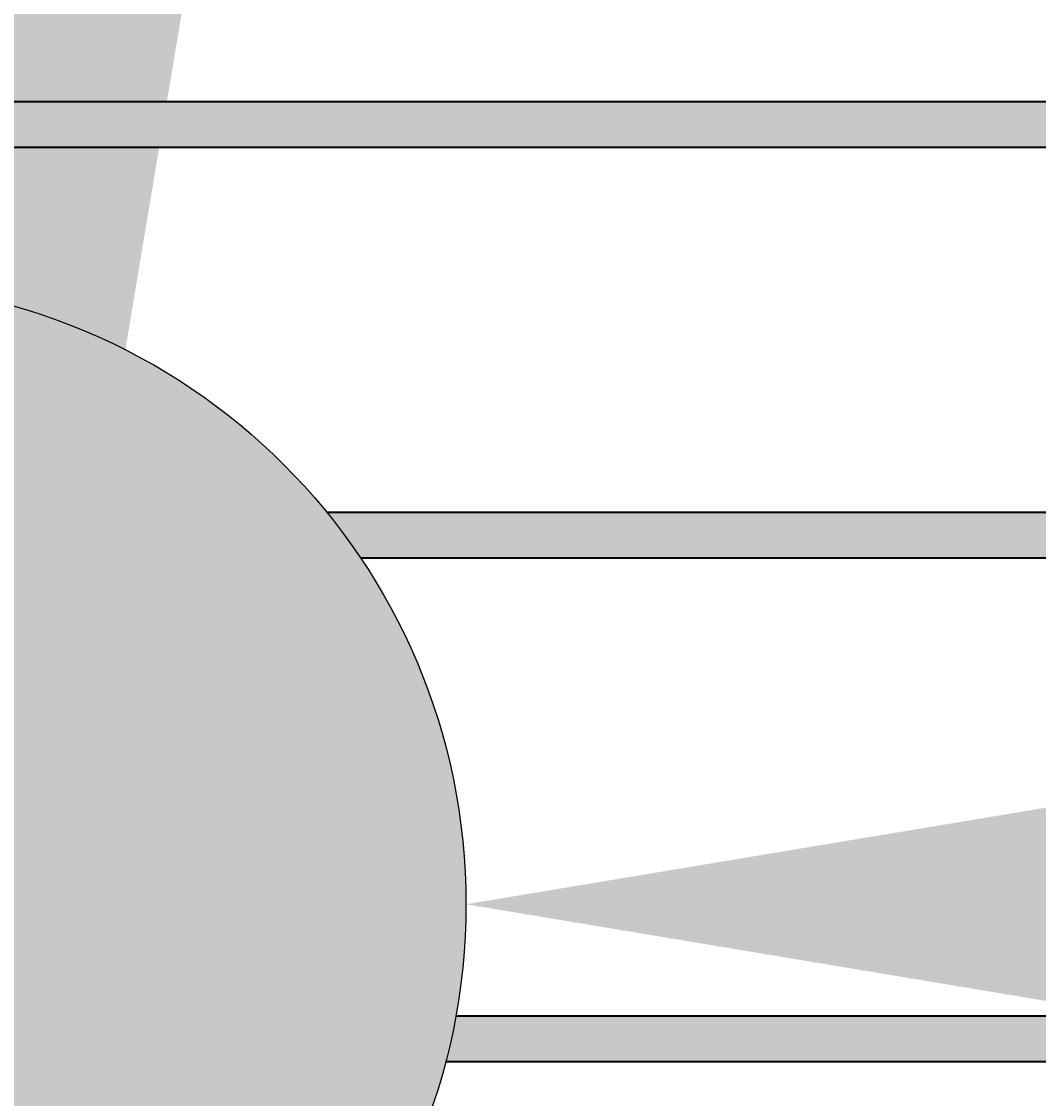
# Model space of a CAD drawing. Units: millimetres. Extents: x -22994 to 29398, y -19990 to 20176.
# Tile 19 of 135: x 54 to 77, y 76 to 99. Entities that reach past the tile are written whole.
import ezdxf

# ---------------------------------------------------------------- set-up
doc = ezdxf.new("R2010")
doc.units = ezdxf.units.MM
doc.header["$MEASUREMENT"] = 0
for name, color, linetype, lineweight in [('M-DIMS', 2, 'Continuous', 18), ('M-EQPM', 7, 'Continuous', 25), ('M-EQPM-PATT', 7, 'Continuous', 18), ('M-PIPE', 7, 'Continuous', 35)]:
    doc.layers.add(name, color=color, linetype=linetype, lineweight=lineweight)
doc.styles.get("Standard").update_dxf_attribs({"font": 'arial.ttf'})
doc.dimstyles.get("Standard").update_dxf_attribs({"dimtxt": 0.18, "dimasz": 10000, "dimexe": 0.18, "dimexo": 0.0625, "dimgap": 0.09, "dimtad": 0, "dimtih": 1, "dimtoh": 1, "dimdec": 0, "dimzin": 0, "dimdsep": 46, "dimtxsty": 'Standard', "dimcen": 0.09, "dimadec": 0, "dimazin": 0, "dimtfac": 1, "dimtdec": 0, "dimtofl": 0, "dimtmove": 0, "dimatfit": 3, "dimfxl": 1, "dimtolj": 1, "dimtzin": 0, "dimlwd": 30, "dimarcsym": 0})

# ---------------------------------------------------------------- blocks, each defined once
blk = doc.blocks.new('*D2')
at = {"layer": 'Defpoints', "color": 0, "transparency": 16777216}
for p in [(6.677, 10.271), (290.852, 10.271), (290.852, -5.079)]:
    blk.add_point(p, dxfattribs=at)
at = {"layer": 'M-DIMS', "color": 0, "lineweight": -2, "transparency": 16777216}
for p, q in [((6.677, 10.209), (6.677, -5.259)), ((290.852, 10.209), (290.852, -5.259))]:
    blk.add_line(p, q, dxfattribs=at)
at = {"layer": 'M-DIMS', "color": 0, "lineweight": 30, "transparency": 16777216}
for p, q in [((-9993.323, -5.079), (-19993.323, -5.079)), ((10290.852, -5.079), (20290.852, -5.079))]:
    blk.add_line(p, q, dxfattribs=at)
at = {"layer": 'M-DIMS', "color": 0, "transparency": 16777216}
for points in [[(-9993.323, 1661.588), (-9993.323, -1671.745), (6.677, -5.079)], [(10290.852, 1661.588), (10290.852, -1671.745), (290.852, -5.079)]]:
    blk.add_solid(points, dxfattribs=at)
at = {"layer": 'M-DIMS', "color": 0, "transparency": 16777216, "insert": (148.765, -5.079), "char_height": 0.18, "attachment_point": 5}
blk.add_mtext('\\A1;284.2', dxfattribs=at)
blk = doc.blocks.new('*D3')
at = {"layer": 'Defpoints', "color": 0, "transparency": 16777216}
for p in [(110.265, 204.165), (110.265, 176.366), (95.833, 127.967)]:
    blk.add_point(p, dxfattribs=at)
at = {"layer": 'M-DIMS', "color": 0, "lineweight": -2, "transparency": 16777216}
for p, q in [((95.833, 128.03), (95.833, 204.345)), ((110.265, 176.429), (110.265, 204.345))]:
    blk.add_line(p, q, dxfattribs=at)
at = {"layer": 'M-DIMS', "color": 0, "lineweight": 30, "transparency": 16777216}
for p, q in [((-9904.167, 204.165), (-19904.167, 204.165)), ((10110.265, 204.165), (20110.265, 204.165))]:
    blk.add_line(p, q, dxfattribs=at)
at = {"layer": 'M-DIMS', "color": 0, "transparency": 16777216}
for points in [[(-9904.167, 1870.832), (-9904.167, -1462.501), (95.833, 204.165)], [(10110.265, 1870.832), (10110.265, -1462.501), (110.265, 204.165)]]:
    blk.add_solid(points, dxfattribs=at)
at = {"layer": 'M-DIMS', "color": 0, "transparency": 16777216, "insert": (103.049, 204.165), "char_height": 0.18, "attachment_point": 5}
blk.add_mtext('\\A1;14.432', dxfattribs=at)
blk = doc.blocks.new('*D4')
at = {"layer": 'Defpoints', "color": 0, "transparency": 16777216}
for p in [(116.265, 204.165), (110.265, 176.366), (116.265, 176.366)]:
    blk.add_point(p, dxfattribs=at)
at = {"layer": 'M-DIMS', "color": 0, "lineweight": -2, "transparency": 16777216}
for p, q in [((110.265, 176.429), (110.265, 204.345)), ((116.265, 176.429), (116.265, 204.345))]:
    blk.add_line(p, q, dxfattribs=at)
at = {"layer": 'M-DIMS', "color": 0, "lineweight": 30, "transparency": 16777216}
for p, q in [((-9889.735, 204.165), (-19889.735, 204.165)), ((10116.265, 204.165), (20116.265, 204.165))]:
    blk.add_line(p, q, dxfattribs=at)
at = {"layer": 'M-DIMS', "color": 0, "transparency": 16777216}
for points in [[(-9889.735, 1870.832), (-9889.735, -1462.501), (110.265, 204.165)], [(10116.265, 1870.832), (10116.265, -1462.501), (116.265, 204.165)]]:
    blk.add_solid(points, dxfattribs=at)
at = {"layer": 'M-DIMS', "color": 0, "transparency": 16777216, "insert": (113.265, 204.165), "char_height": 0.18, "attachment_point": 5}
blk.add_mtext('\\A1;6', dxfattribs=at)
blk = doc.blocks.new('*D5')
at = {"layer": 'Defpoints', "color": 0, "transparency": 16777216}
for p in [(181.265, 204.165), (116.265, 176.366), (181.265, 176.366)]:
    blk.add_point(p, dxfattribs=at)
at = {"layer": 'M-DIMS', "color": 0, "lineweight": -2, "transparency": 16777216}
for p, q in [((116.265, 176.429), (116.265, 204.345)), ((181.265, 176.429), (181.265, 204.345))]:
    blk.add_line(p, q, dxfattribs=at)
at = {"layer": 'M-DIMS', "color": 0, "lineweight": 30, "transparency": 16777216}
for p, q in [((-9883.735, 204.165), (-19883.735, 204.165)), ((10181.265, 204.165), (20181.265, 204.165))]:
    blk.add_line(p, q, dxfattribs=at)
at = {"layer": 'M-DIMS', "color": 0, "transparency": 16777216}
for points in [[(-9883.735, 1870.832), (-9883.735, -1462.501), (116.265, 204.165)], [(10181.265, 1870.832), (10181.265, -1462.501), (181.265, 204.165)]]:
    blk.add_solid(points, dxfattribs=at)
at = {"layer": 'M-DIMS', "color": 0, "transparency": 16777216, "insert": (148.765, 204.165), "char_height": 0.18, "attachment_point": 5}
blk.add_mtext('\\A1;65', dxfattribs=at)
blk = doc.blocks.new('*D6')
at = {"layer": 'Defpoints', "color": 0, "transparency": 16777216}
for p in [(187.265, 204.165), (181.265, 176.366), (187.265, 176.366)]:
    blk.add_point(p, dxfattribs=at)
at = {"layer": 'M-DIMS', "color": 0, "lineweight": -2, "transparency": 16777216}
for p, q in [((181.265, 176.429), (181.265, 204.345)), ((187.265, 176.429), (187.265, 204.345))]:
    blk.add_line(p, q, dxfattribs=at)
at = {"layer": 'M-DIMS', "color": 0, "lineweight": 30, "transparency": 16777216}
for p, q in [((-9818.735, 204.165), (-19818.735, 204.165)), ((10187.265, 204.165), (20187.265, 204.165))]:
    blk.add_line(p, q, dxfattribs=at)
at = {"layer": 'M-DIMS', "color": 0, "transparency": 16777216}
for points in [[(-9818.735, 1870.832), (-9818.735, -1462.501), (181.265, 204.165)], [(10187.265, 1870.832), (10187.265, -1462.501), (187.265, 204.165)]]:
    blk.add_solid(points, dxfattribs=at)
at = {"layer": 'M-DIMS', "color": 0, "transparency": 16777216, "insert": (184.265, 204.165), "char_height": 0.18, "attachment_point": 5}
blk.add_mtext('\\A1;6', dxfattribs=at)
blk = doc.blocks.new('*D7')
at = {"layer": 'Defpoints', "color": 0, "transparency": 16777216}
for p in [(201.697, 204.165), (187.265, 176.366), (201.697, 127.967)]:
    blk.add_point(p, dxfattribs=at)
at = {"layer": 'M-DIMS', "color": 0, "lineweight": -2, "transparency": 16777216}
for p, q in [((187.265, 176.429), (187.265, 204.345)), ((201.697, 128.03), (201.697, 204.345))]:
    blk.add_line(p, q, dxfattribs=at)
at = {"layer": 'M-DIMS', "color": 0, "lineweight": 30, "transparency": 16777216}
for p, q in [((-9812.735, 204.165), (-19812.735, 204.165)), ((10201.697, 204.165), (20201.697, 204.165))]:
    blk.add_line(p, q, dxfattribs=at)
at = {"layer": 'M-DIMS', "color": 0, "transparency": 16777216}
for points in [[(-9812.735, 1870.832), (-9812.735, -1462.501), (187.265, 204.165)], [(10201.697, 1870.832), (10201.697, -1462.501), (201.697, 204.165)]]:
    blk.add_solid(points, dxfattribs=at)
at = {"layer": 'M-DIMS', "color": 0, "transparency": 16777216, "insert": (194.481, 204.165), "char_height": 0.18, "attachment_point": 5}
blk.add_mtext('\\A1;14.432', dxfattribs=at)
blk = doc.blocks.new('*D8')
at = {"layer": 'Defpoints', "color": 0, "transparency": 16777216}
for p in [(227.648, 204.165), (227.648, 146.73), (201.697, 127.967)]:
    blk.add_point(p, dxfattribs=at)
at = {"layer": 'M-DIMS', "color": 0, "lineweight": -2, "transparency": 16777216}
for p, q in [((201.697, 128.03), (201.697, 204.345)), ((227.648, 146.792), (227.648, 204.345))]:
    blk.add_line(p, q, dxfattribs=at)
at = {"layer": 'M-DIMS', "color": 0, "lineweight": 30, "transparency": 16777216}
for p, q in [((-9798.303, 204.165), (-19798.303, 204.165)), ((10227.648, 204.165), (20227.648, 204.165))]:
    blk.add_line(p, q, dxfattribs=at)
at = {"layer": 'M-DIMS', "color": 0, "transparency": 16777216}
for points in [[(-9798.303, 1870.832), (-9798.303, -1462.501), (201.697, 204.165)], [(10227.648, 1870.832), (10227.648, -1462.501), (227.648, 204.165)]]:
    blk.add_solid(points, dxfattribs=at)
at = {"layer": 'M-DIMS', "color": 0, "transparency": 16777216, "insert": (214.673, 204.165), "char_height": 0.18, "attachment_point": 5}
blk.add_mtext('\\A1;25.95', dxfattribs=at)
blk = doc.blocks.new('*D9')
at = {"layer": 'Defpoints', "color": 0, "transparency": 16777216}
for p in [(187.265, 176.366), (306.202, 176.366), (290.852, 10.271)]:
    blk.add_point(p, dxfattribs=at)
at = {"layer": 'M-DIMS', "color": 0, "lineweight": 30, "transparency": 16777216}
for p, q in [((306.202, 10176.366), (306.202, 20176.366)), ((306.202, -9989.729), (306.202, -19989.729))]:
    blk.add_line(p, q, dxfattribs=at)
at = {"layer": 'M-DIMS', "color": 0, "lineweight": -2, "transparency": 16777216}
for p, q in [((187.327, 176.366), (306.382, 176.366)), ((290.915, 10.271), (306.382, 10.271))]:
    blk.add_line(p, q, dxfattribs=at)
at = {"layer": 'M-DIMS', "color": 0, "transparency": 16777216}
for points in [[(-1360.465, 10176.366), (1972.869, 10176.366), (306.202, 176.366)], [(-1360.465, -9989.729), (1972.869, -9989.729), (306.202, 10.271)]]:
    blk.add_solid(points, dxfattribs=at)
at = {"layer": 'M-DIMS', "color": 0, "transparency": 16777216, "insert": (306.202, 93.319), "char_height": 0.18, "attachment_point": 5}
blk.add_mtext('\\A1;166.1', dxfattribs=at)
blk = doc.blocks.new('*D10')
at = {"layer": 'Defpoints', "color": 0, "transparency": 16777216}
for p in [(125.65, 136.071), (133.346, 136.071), (133.346, -5.079)]:
    blk.add_point(p, dxfattribs=at)
at = {"layer": 'M-DIMS', "color": 0, "lineweight": -2, "transparency": 16777216}
for p, q in [((125.65, 136.009), (125.65, -5.259)), ((133.346, 136.009), (133.346, -5.259))]:
    blk.add_line(p, q, dxfattribs=at)
at = {"layer": 'M-DIMS', "color": 0, "lineweight": 30, "transparency": 16777216}
for p, q in [((-9874.35, -5.079), (-19874.35, -5.079)), ((10133.346, -5.079), (20133.346, -5.079))]:
    blk.add_line(p, q, dxfattribs=at)
at = {"layer": 'M-DIMS', "color": 0, "transparency": 16777216}
for points in [[(-9874.35, 1661.588), (-9874.35, -1671.745), (125.65, -5.079)], [(10133.346, 1661.588), (10133.346, -1671.745), (133.346, -5.079)]]:
    blk.add_solid(points, dxfattribs=at)
at = {"layer": 'M-DIMS', "color": 0, "transparency": 16777216, "insert": (129.498, -5.079), "char_height": 0.18, "attachment_point": 5}
blk.add_mtext('\\A1;7.696', dxfattribs=at)
blk = doc.blocks.new('*D11')
at = {"layer": 'Defpoints', "color": 0, "transparency": 16777216}
for p in [(133.346, 136.071), (135.65, 136.071), (135.65, -5.079)]:
    blk.add_point(p, dxfattribs=at)
at = {"layer": 'M-DIMS', "color": 0, "lineweight": -2, "transparency": 16777216}
for p, q in [((133.346, 136.009), (133.346, -5.259)), ((135.65, 136.009), (135.65, -5.259))]:
    blk.add_line(p, q, dxfattribs=at)
at = {"layer": 'M-DIMS', "color": 0, "lineweight": 30, "transparency": 16777216}
for p, q in [((-9866.654, -5.079), (-19866.654, -5.079)), ((10135.65, -5.079), (20135.65, -5.079))]:
    blk.add_line(p, q, dxfattribs=at)
at = {"layer": 'M-DIMS', "color": 0, "transparency": 16777216}
for points in [[(-9866.654, 1661.588), (-9866.654, -1671.745), (133.346, -5.079)], [(10135.65, 1661.588), (10135.65, -1671.745), (135.65, -5.079)]]:
    blk.add_solid(points, dxfattribs=at)
at = {"layer": 'M-DIMS', "color": 0, "transparency": 16777216, "insert": (134.498, -5.079), "char_height": 0.18, "attachment_point": 5}
blk.add_mtext('\\A1;2.304', dxfattribs=at)
blk = doc.blocks.new('*D12')
at = {"layer": 'Defpoints', "color": 0, "transparency": 16777216}
for p in [(135.65, 136.071), (145.65, 136.071), (145.65, -5.079)]:
    blk.add_point(p, dxfattribs=at)
at = {"layer": 'M-DIMS', "color": 0, "lineweight": -2, "transparency": 16777216}
for p, q in [((135.65, 136.009), (135.65, -5.259)), ((145.65, 136.009), (145.65, -5.259))]:
    blk.add_line(p, q, dxfattribs=at)
at = {"layer": 'M-DIMS', "color": 0, "lineweight": 30, "transparency": 16777216}
for p, q in [((-9864.35, -5.079), (-19864.35, -5.079)), ((10145.65, -5.079), (20145.65, -5.079))]:
    blk.add_line(p, q, dxfattribs=at)
at = {"layer": 'M-DIMS', "color": 0, "transparency": 16777216}
for points in [[(-9864.35, 1661.588), (-9864.35, -1671.745), (135.65, -5.079)], [(10145.65, 1661.588), (10145.65, -1671.745), (145.65, -5.079)]]:
    blk.add_solid(points, dxfattribs=at)
at = {"layer": 'M-DIMS', "color": 0, "transparency": 16777216, "insert": (140.65, -5.079), "char_height": 0.18, "attachment_point": 5}
blk.add_mtext('\\A1;10', dxfattribs=at)
blk = doc.blocks.new('*D13')
at = {"layer": 'Defpoints', "color": 0, "transparency": 16777216}
for p in [(145.65, 136.071), (155.65, 136.071), (155.65, -5.079)]:
    blk.add_point(p, dxfattribs=at)
at = {"layer": 'M-DIMS', "color": 0, "lineweight": -2, "transparency": 16777216}
for p, q in [((145.65, 136.009), (145.65, -5.259)), ((155.65, 136.009), (155.65, -5.259))]:
    blk.add_line(p, q, dxfattribs=at)
at = {"layer": 'M-DIMS', "color": 0, "lineweight": 30, "transparency": 16777216}
for p, q in [((-9854.35, -5.079), (-19854.35, -5.079)), ((10155.65, -5.079), (20155.65, -5.079))]:
    blk.add_line(p, q, dxfattribs=at)
at = {"layer": 'M-DIMS', "color": 0, "transparency": 16777216}
for points in [[(-9854.35, 1661.588), (-9854.35, -1671.745), (145.65, -5.079)], [(10155.65, 1661.588), (10155.65, -1671.745), (155.65, -5.079)]]:
    blk.add_solid(points, dxfattribs=at)
at = {"layer": 'M-DIMS', "color": 0, "transparency": 16777216, "insert": (150.65, -5.079), "char_height": 0.18, "attachment_point": 5}
blk.add_mtext('\\A1;10', dxfattribs=at)
blk = doc.blocks.new('*D14')
at = {"layer": 'Defpoints', "color": 0, "transparency": 16777216}
for p in [(155.65, 136.071), (165.65, 136.071), (165.65, -5.079)]:
    blk.add_point(p, dxfattribs=at)
at = {"layer": 'M-DIMS', "color": 0, "lineweight": -2, "transparency": 16777216}
for p, q in [((155.65, 136.009), (155.65, -5.259)), ((165.65, 136.009), (165.65, -5.259))]:
    blk.add_line(p, q, dxfattribs=at)
at = {"layer": 'M-DIMS', "color": 0, "lineweight": 30, "transparency": 16777216}
for p, q in [((-9844.35, -5.079), (-19844.35, -5.079)), ((10165.65, -5.079), (20165.65, -5.079))]:
    blk.add_line(p, q, dxfattribs=at)
at = {"layer": 'M-DIMS', "color": 0, "transparency": 16777216}
for points in [[(-9844.35, 1661.588), (-9844.35, -1671.745), (155.65, -5.079)], [(10165.65, 1661.588), (10165.65, -1671.745), (165.65, -5.079)]]:
    blk.add_solid(points, dxfattribs=at)
at = {"layer": 'M-DIMS', "color": 0, "transparency": 16777216, "insert": (160.65, -5.079), "char_height": 0.18, "attachment_point": 5}
blk.add_mtext('\\A1;10', dxfattribs=at)
blk = doc.blocks.new('*D15')
at = {"layer": 'Defpoints', "color": 0, "transparency": 16777216}
for p in [(173.346, 154.788), (173.346, 136.071), (306.202, 136.071)]:
    blk.add_point(p, dxfattribs=at)
at = {"layer": 'M-DIMS', "color": 0, "lineweight": 30, "transparency": 16777216}
for p, q in [((306.202, 10154.788), (306.202, 20154.788)), ((306.202, -9863.929), (306.202, -19863.929))]:
    blk.add_line(p, q, dxfattribs=at)
at = {"layer": 'M-DIMS', "color": 0, "lineweight": -2, "transparency": 16777216}
for p, q in [((173.408, 154.788), (306.382, 154.788)), ((173.408, 136.071), (306.382, 136.071))]:
    blk.add_line(p, q, dxfattribs=at)
at = {"layer": 'M-DIMS', "color": 0, "transparency": 16777216}
for points in [[(-1360.465, 10154.788), (1972.869, 10154.788), (306.202, 154.788)], [(-1360.465, -9863.929), (1972.869, -9863.929), (306.202, 136.071)]]:
    blk.add_solid(points, dxfattribs=at)
at = {"layer": 'M-DIMS', "color": 0, "transparency": 16777216, "insert": (306.202, 145.43), "char_height": 0.18, "attachment_point": 5}
blk.add_mtext('\\A1;18.717', dxfattribs=at)
blk = doc.blocks.new('*D16')
at = {"layer": 'Defpoints', "color": 0, "transparency": 16777216}
for p in [(120.17, 204.165), (110.466, 48.035), (120.17, 48.035)]:
    blk.add_point(p, dxfattribs=at)
at = {"layer": 'M-DIMS', "color": 0, "lineweight": -2, "transparency": 16777216}
for p, q in [((110.466, 48.097), (110.466, 204.345)), ((120.17, 48.097), (120.17, 204.345))]:
    blk.add_line(p, q, dxfattribs=at)
at = {"layer": 'M-DIMS', "color": 0, "lineweight": 30, "transparency": 16777216}
for p, q in [((-9889.534, 204.165), (-19889.534, 204.165)), ((10120.17, 204.165), (20120.17, 204.165))]:
    blk.add_line(p, q, dxfattribs=at)
at = {"layer": 'M-DIMS', "color": 0, "transparency": 16777216}
for points in [[(-9889.534, 1870.832), (-9889.534, -1462.501), (110.466, 204.165)], [(10120.17, 1870.832), (10120.17, -1462.501), (120.17, 204.165)]]:
    blk.add_solid(points, dxfattribs=at)
at = {"layer": 'M-DIMS', "color": 0, "transparency": 16777216, "insert": (115.318, 204.165), "char_height": 0.18, "attachment_point": 5}
blk.add_mtext('\\A1;9.704', dxfattribs=at)
blk = doc.blocks.new('*D17')
at = {"layer": 'Defpoints', "color": 0, "transparency": 16777216}
for p in [(126.17, 204.165), (120.17, 48.035), (126.17, 48.035)]:
    blk.add_point(p, dxfattribs=at)
at = {"layer": 'M-DIMS', "color": 0, "lineweight": -2, "transparency": 16777216}
for p, q in [((120.17, 48.097), (120.17, 204.345)), ((126.17, 48.097), (126.17, 204.345))]:
    blk.add_line(p, q, dxfattribs=at)
at = {"layer": 'M-DIMS', "color": 0, "lineweight": 30, "transparency": 16777216}
for p, q in [((-9879.83, 204.165), (-19879.83, 204.165)), ((10126.17, 204.165), (20126.17, 204.165))]:
    blk.add_line(p, q, dxfattribs=at)
at = {"layer": 'M-DIMS', "color": 0, "transparency": 16777216}
for points in [[(-9879.83, 1870.832), (-9879.83, -1462.501), (120.17, 204.165)], [(10126.17, 1870.832), (10126.17, -1462.501), (126.17, 204.165)]]:
    blk.add_solid(points, dxfattribs=at)
at = {"layer": 'M-DIMS', "color": 0, "transparency": 16777216, "insert": (123.17, 204.165), "char_height": 0.18, "attachment_point": 5}
blk.add_mtext('\\A1;6', dxfattribs=at)
blk = doc.blocks.new('*D18')
at = {"layer": 'Defpoints', "color": 0, "transparency": 16777216}
for p in [(132.17, 204.165), (126.17, 48.035), (132.17, 48.035)]:
    blk.add_point(p, dxfattribs=at)
at = {"layer": 'M-DIMS', "color": 0, "lineweight": -2, "transparency": 16777216}
for p, q in [((126.17, 48.097), (126.17, 204.345)), ((132.17, 48.097), (132.17, 204.345))]:
    blk.add_line(p, q, dxfattribs=at)
at = {"layer": 'M-DIMS', "color": 0, "lineweight": 30, "transparency": 16777216}
for p, q in [((-9873.83, 204.165), (-19873.83, 204.165)), ((10132.17, 204.165), (20132.17, 204.165))]:
    blk.add_line(p, q, dxfattribs=at)
at = {"layer": 'M-DIMS', "color": 0, "transparency": 16777216}
for points in [[(-9873.83, 1870.832), (-9873.83, -1462.501), (126.17, 204.165)], [(10132.17, 1870.832), (10132.17, -1462.501), (132.17, 204.165)]]:
    blk.add_solid(points, dxfattribs=at)
at = {"layer": 'M-DIMS', "color": 0, "transparency": 16777216, "insert": (129.17, 204.165), "char_height": 0.18, "attachment_point": 5}
blk.add_mtext('\\A1;6', dxfattribs=at)
blk = doc.blocks.new('*D19')
at = {"layer": 'Defpoints', "color": 0, "transparency": 16777216}
for p in [(138.17, 204.165), (132.17, 48.035), (138.17, 48.035)]:
    blk.add_point(p, dxfattribs=at)
at = {"layer": 'M-DIMS', "color": 0, "lineweight": -2, "transparency": 16777216}
for p, q in [((132.17, 48.097), (132.17, 204.345)), ((138.17, 48.097), (138.17, 204.345))]:
    blk.add_line(p, q, dxfattribs=at)
at = {"layer": 'M-DIMS', "color": 0, "lineweight": 30, "transparency": 16777216}
for p, q in [((-9867.83, 204.165), (-19867.83, 204.165)), ((10138.17, 204.165), (20138.17, 204.165))]:
    blk.add_line(p, q, dxfattribs=at)
at = {"layer": 'M-DIMS', "color": 0, "transparency": 16777216}
for points in [[(-9867.83, 1870.832), (-9867.83, -1462.501), (132.17, 204.165)], [(10138.17, 1870.832), (10138.17, -1462.501), (138.17, 204.165)]]:
    blk.add_solid(points, dxfattribs=at)
at = {"layer": 'M-DIMS', "color": 0, "transparency": 16777216, "insert": (135.17, 204.165), "char_height": 0.18, "attachment_point": 5}
blk.add_mtext('\\A1;6', dxfattribs=at)
blk = doc.blocks.new('*D20')
at = {"layer": 'Defpoints', "color": 0, "transparency": 16777216}
for p in [(144.17, 204.165), (138.17, 48.035), (144.17, 48.035)]:
    blk.add_point(p, dxfattribs=at)
at = {"layer": 'M-DIMS', "color": 0, "lineweight": -2, "transparency": 16777216}
for p, q in [((138.17, 48.097), (138.17, 204.345)), ((144.17, 48.097), (144.17, 204.345))]:
    blk.add_line(p, q, dxfattribs=at)
at = {"layer": 'M-DIMS', "color": 0, "lineweight": 30, "transparency": 16777216}
for p, q in [((-9861.83, 204.165), (-19861.83, 204.165)), ((10144.17, 204.165), (20144.17, 204.165))]:
    blk.add_line(p, q, dxfattribs=at)
at = {"layer": 'M-DIMS', "color": 0, "transparency": 16777216}
for points in [[(-9861.83, 1870.832), (-9861.83, -1462.501), (138.17, 204.165)], [(10144.17, 1870.832), (10144.17, -1462.501), (144.17, 204.165)]]:
    blk.add_solid(points, dxfattribs=at)
at = {"layer": 'M-DIMS', "color": 0, "transparency": 16777216, "insert": (141.17, 204.165), "char_height": 0.18, "attachment_point": 5}
blk.add_mtext('\\A1;6', dxfattribs=at)
blk = doc.blocks.new('*D21')
at = {"layer": 'Defpoints', "color": 0, "transparency": 16777216}
for p in [(149.116, 204.165), (144.17, 48.035), (149.116, 48.035)]:
    blk.add_point(p, dxfattribs=at)
at = {"layer": 'M-DIMS', "color": 0, "lineweight": -2, "transparency": 16777216}
for p, q in [((144.17, 48.097), (144.17, 204.345)), ((149.116, 48.097), (149.116, 204.345))]:
    blk.add_line(p, q, dxfattribs=at)
at = {"layer": 'M-DIMS', "color": 0, "lineweight": 30, "transparency": 16777216}
for p, q in [((-9855.83, 204.165), (-19855.83, 204.165)), ((10149.116, 204.165), (20149.116, 204.165))]:
    blk.add_line(p, q, dxfattribs=at)
at = {"layer": 'M-DIMS', "color": 0, "transparency": 16777216}
for points in [[(-9855.83, 1870.832), (-9855.83, -1462.501), (144.17, 204.165)], [(10149.116, 1870.832), (10149.116, -1462.501), (149.116, 204.165)]]:
    blk.add_solid(points, dxfattribs=at)
at = {"layer": 'M-DIMS', "color": 0, "transparency": 16777216, "insert": (146.643, 204.165), "char_height": 0.18, "attachment_point": 5}
blk.add_mtext('\\A1;4.945', dxfattribs=at)
blk = doc.blocks.new('*D22')
at = {"layer": 'Defpoints', "color": 0, "transparency": 16777216}
for p in [(149.116, 30.99), (155.116, 30.99), (155.116, -5.079)]:
    blk.add_point(p, dxfattribs=at)
at = {"layer": 'M-DIMS', "color": 0, "lineweight": -2, "transparency": 16777216}
for p, q in [((149.116, 30.927), (149.116, -5.259)), ((155.116, 30.927), (155.116, -5.259))]:
    blk.add_line(p, q, dxfattribs=at)
at = {"layer": 'M-DIMS', "color": 0, "lineweight": 30, "transparency": 16777216}
for p, q in [((-9850.884, -5.079), (-19850.884, -5.079)), ((10155.116, -5.079), (20155.116, -5.079))]:
    blk.add_line(p, q, dxfattribs=at)
at = {"layer": 'M-DIMS', "color": 0, "transparency": 16777216}
for points in [[(-9850.884, 1661.588), (-9850.884, -1671.745), (149.116, -5.079)], [(10155.116, 1661.588), (10155.116, -1671.745), (155.116, -5.079)]]:
    blk.add_solid(points, dxfattribs=at)
at = {"layer": 'M-DIMS', "color": 0, "transparency": 16777216, "insert": (152.116, -5.079), "char_height": 0.18, "attachment_point": 5}
blk.add_mtext('\\A1;6', dxfattribs=at)
blk = doc.blocks.new('*D23')
at = {"layer": 'Defpoints', "color": 0, "transparency": 16777216}
for p in [(155.116, 30.99), (161.116, 30.99), (161.116, -5.079)]:
    blk.add_point(p, dxfattribs=at)
at = {"layer": 'M-DIMS', "color": 0, "lineweight": -2, "transparency": 16777216}
for p, q in [((155.116, 30.927), (155.116, -5.259)), ((161.116, 30.927), (161.116, -5.259))]:
    blk.add_line(p, q, dxfattribs=at)
at = {"layer": 'M-DIMS', "color": 0, "lineweight": 30, "transparency": 16777216}
for p, q in [((-9844.884, -5.079), (-19844.884, -5.079)), ((10161.116, -5.079), (20161.116, -5.079))]:
    blk.add_line(p, q, dxfattribs=at)
at = {"layer": 'M-DIMS', "color": 0, "transparency": 16777216}
for points in [[(-9844.884, 1661.588), (-9844.884, -1671.745), (155.116, -5.079)], [(10161.116, 1661.588), (10161.116, -1671.745), (161.116, -5.079)]]:
    blk.add_solid(points, dxfattribs=at)
at = {"layer": 'M-DIMS', "color": 0, "transparency": 16777216, "insert": (158.116, -5.079), "char_height": 0.18, "attachment_point": 5}
blk.add_mtext('\\A1;6', dxfattribs=at)
blk = doc.blocks.new('*D24')
at = {"layer": 'Defpoints', "color": 0, "transparency": 16777216}
for p in [(161.116, 30.99), (166.439, 30.99), (166.439, -5.079)]:
    blk.add_point(p, dxfattribs=at)
at = {"layer": 'M-DIMS', "color": 0, "lineweight": -2, "transparency": 16777216}
for p, q in [((161.116, 30.927), (161.116, -5.259)), ((166.439, 30.927), (166.439, -5.259))]:
    blk.add_line(p, q, dxfattribs=at)
at = {"layer": 'M-DIMS', "color": 0, "lineweight": 30, "transparency": 16777216}
for p, q in [((-9838.884, -5.079), (-19838.884, -5.079)), ((10166.439, -5.079), (20166.439, -5.079))]:
    blk.add_line(p, q, dxfattribs=at)
at = {"layer": 'M-DIMS', "color": 0, "transparency": 16777216}
for points in [[(-9838.884, 1661.588), (-9838.884, -1671.745), (161.116, -5.079)], [(10166.439, 1661.588), (10166.439, -1671.745), (166.439, -5.079)]]:
    blk.add_solid(points, dxfattribs=at)
at = {"layer": 'M-DIMS', "color": 0, "transparency": 16777216, "insert": (163.777, -5.079), "char_height": 0.18, "attachment_point": 5}
blk.add_mtext('\\A1;5.323', dxfattribs=at)
blk = doc.blocks.new('*D25')
at = {"layer": 'Defpoints', "color": 0, "transparency": 16777216}
for p in [(166.439, 30.99), (172.439, 30.99), (172.439, -5.079)]:
    blk.add_point(p, dxfattribs=at)
at = {"layer": 'M-DIMS', "color": 0, "lineweight": -2, "transparency": 16777216}
for p, q in [((166.439, 30.927), (166.439, -5.259)), ((172.439, 30.927), (172.439, -5.259))]:
    blk.add_line(p, q, dxfattribs=at)
at = {"layer": 'M-DIMS', "color": 0, "lineweight": 30, "transparency": 16777216}
for p, q in [((-9833.561, -5.079), (-19833.561, -5.079)), ((10172.439, -5.079), (20172.439, -5.079))]:
    blk.add_line(p, q, dxfattribs=at)
at = {"layer": 'M-DIMS', "color": 0, "transparency": 16777216}
for points in [[(-9833.561, 1661.588), (-9833.561, -1671.745), (166.439, -5.079)], [(10172.439, 1661.588), (10172.439, -1671.745), (172.439, -5.079)]]:
    blk.add_solid(points, dxfattribs=at)
at = {"layer": 'M-DIMS', "color": 0, "transparency": 16777216, "insert": (169.439, -5.079), "char_height": 0.18, "attachment_point": 5}
blk.add_mtext('\\A1;6', dxfattribs=at)
blk = doc.blocks.new('*D26')
at = {"layer": 'Defpoints', "color": 0, "transparency": 16777216}
for p in [(172.439, 30.99), (178.439, 30.99), (178.439, -5.079)]:
    blk.add_point(p, dxfattribs=at)
at = {"layer": 'M-DIMS', "color": 0, "lineweight": -2, "transparency": 16777216}
for p, q in [((172.439, 30.927), (172.439, -5.259)), ((178.439, 30.927), (178.439, -5.259))]:
    blk.add_line(p, q, dxfattribs=at)
at = {"layer": 'M-DIMS', "color": 0, "lineweight": 30, "transparency": 16777216}
for p, q in [((-9827.561, -5.079), (-19827.561, -5.079)), ((10178.439, -5.079), (20178.439, -5.079))]:
    blk.add_line(p, q, dxfattribs=at)
at = {"layer": 'M-DIMS', "color": 0, "transparency": 16777216}
for points in [[(-9827.561, 1661.588), (-9827.561, -1671.745), (172.439, -5.079)], [(10178.439, 1661.588), (10178.439, -1671.745), (178.439, -5.079)]]:
    blk.add_solid(points, dxfattribs=at)
at = {"layer": 'M-DIMS', "color": 0, "transparency": 16777216, "insert": (175.439, -5.079), "char_height": 0.18, "attachment_point": 5}
blk.add_mtext('\\A1;6', dxfattribs=at)
blk = doc.blocks.new('*D27')
at = {"layer": 'Defpoints', "color": 0, "transparency": 16777216}
for p in [(178.439, 30.99), (188.117, 30.99), (188.117, -5.079)]:
    blk.add_point(p, dxfattribs=at)
at = {"layer": 'M-DIMS', "color": 0, "lineweight": -2, "transparency": 16777216}
for p, q in [((178.439, 30.927), (178.439, -5.259)), ((188.117, 30.927), (188.117, -5.259))]:
    blk.add_line(p, q, dxfattribs=at)
at = {"layer": 'M-DIMS', "color": 0, "lineweight": 30, "transparency": 16777216}
for p, q in [((-9821.561, -5.079), (-19821.561, -5.079)), ((10188.117, -5.079), (20188.117, -5.079))]:
    blk.add_line(p, q, dxfattribs=at)
at = {"layer": 'M-DIMS', "color": 0, "transparency": 16777216}
for points in [[(-9821.561, 1661.588), (-9821.561, -1671.745), (178.439, -5.079)], [(10188.117, 1661.588), (10188.117, -1671.745), (188.117, -5.079)]]:
    blk.add_solid(points, dxfattribs=at)
at = {"layer": 'M-DIMS', "color": 0, "transparency": 16777216, "insert": (183.278, -5.079), "char_height": 0.18, "attachment_point": 5}
blk.add_mtext('\\A1;9.679', dxfattribs=at)
blk = doc.blocks.new('*D28')
at = {"layer": 'Defpoints', "color": 0, "transparency": 16777216}
for p in [(188.117, 48.035), (306.202, 48.035), (188.117, 30.99)]:
    blk.add_point(p, dxfattribs=at)
at = {"layer": 'M-DIMS', "color": 0, "lineweight": 30, "transparency": 16777216}
for p, q in [((306.202, 10048.035), (306.202, 20048.035)), ((306.202, -9969.01), (306.202, -19969.01))]:
    blk.add_line(p, q, dxfattribs=at)
at = {"layer": 'M-DIMS', "color": 0, "lineweight": -2, "transparency": 16777216}
for p, q in [((188.18, 48.035), (306.382, 48.035)), ((188.18, 30.99), (306.382, 30.99))]:
    blk.add_line(p, q, dxfattribs=at)
at = {"layer": 'M-DIMS', "color": 0, "transparency": 16777216}
for points in [[(-1360.465, 10048.035), (1972.869, 10048.035), (306.202, 48.035)], [(-1360.465, -9969.01), (1972.869, -9969.01), (306.202, 30.99)]]:
    blk.add_solid(points, dxfattribs=at)
at = {"layer": 'M-DIMS', "color": 0, "transparency": 16777216, "insert": (306.202, 39.512), "char_height": 0.18, "attachment_point": 5}
blk.add_mtext('\\A1;17.045', dxfattribs=at)
blk = doc.blocks.new('*D29')
at = {"layer": 'Defpoints', "color": 0, "transparency": 16777216}
for p in [(36.801, 80.045), (64.03, 80.045)]:
    blk.add_point(p, dxfattribs=at)
at = {"layer": 'M-DIMS', "color": 0, "lineweight": -2, "transparency": 16777216}
for p, q in [((50.325, 80.045), (50.505, 80.045)), ((50.415, 79.955), (50.415, 80.135))]:
    blk.add_line(p, q, dxfattribs=at)
at = {"layer": 'M-DIMS', "color": 0, "lineweight": 30, "transparency": 16777216}
blk.add_line((20064.03, 80.03), (10064.03, 80.038), dxfattribs=at)
at = {"layer": 'M-DIMS', "color": 0, "transparency": 16777216}
blk.add_solid([(10064.031, 1746.704), (10064.028, -1586.629), (64.03, 80.045)], dxfattribs=at)
at = {"layer": 'M-DIMS', "color": 0, "transparency": 16777216, "insert": (20064.521, 80.03), "char_height": 0.18, "attachment_point": 5}
blk.add_mtext('\\A1;∅27.23', dxfattribs=at)
blk = doc.blocks.new('*D32')
at = {"layer": 'Defpoints', "color": 0, "transparency": 16777216}
for p in [(57.164, 118.614), (52.413, 113.093)]:
    blk.add_point(p, dxfattribs=at)
at = {"layer": 'M-DIMS', "color": 0, "lineweight": -2, "transparency": 16777216}
for p, q in [((57.164, 118.524), (57.164, 118.704)), ((57.074, 118.614), (57.254, 118.614))]:
    blk.add_line(p, q, dxfattribs=at)
at = {"layer": 'M-DIMS', "color": 0, "lineweight": 30, "transparency": 16777216}
for p, q in [((-12992.534, -15047.031), (-6470.06, -7466.969)), ((-22992.534, -15047.031), (-12992.534, -15047.031))]:
    blk.add_line(p, q, dxfattribs=at)
at = {"layer": 'M-DIMS', "color": 0, "transparency": 16777216}
blk.add_solid([(-7733.404, -6379.89), (-5206.717, -8554.048), (52.413, 113.093)], dxfattribs=at)
at = {"layer": 'M-DIMS', "color": 0, "transparency": 16777216, "insert": (-22993.208, -15047.031), "char_height": 0.18, "attachment_point": 5}
blk.add_mtext('\\A1;2X R7.284', dxfattribs=at)
blk = doc.blocks.new('*D36')
at = {"layer": 'Defpoints', "color": 0, "transparency": 16777216}
for p in [(46.39, 31.303), (46.387, 26.593)]:
    blk.add_point(p, dxfattribs=at)
at = {"layer": 'M-DIMS', "color": 0, "lineweight": 30, "transparency": 16777216}
for p, q in [((57.15, 20031.301), (51.77, 10031.302)), ((10057.15, 20031.301), (57.15, 20031.301))]:
    blk.add_line(p, q, dxfattribs=at)
at = {"layer": 'M-DIMS', "color": 0, "lineweight": -2, "transparency": 16777216}
for p, q in [((46.389, 28.858), (46.389, 29.038)), ((46.299, 28.948), (46.479, 28.948))]:
    blk.add_line(p, q, dxfattribs=at)
at = {"layer": 'M-DIMS', "color": 0, "transparency": 16777216}
blk.add_solid([(-1614.896, 10032.199), (1718.436, 10030.405), (46.39, 31.303)], dxfattribs=at)
at = {"layer": 'M-DIMS', "color": 0, "transparency": 16777216, "insert": (10057.554, 20031.301), "char_height": 0.18, "attachment_point": 5}
blk.add_mtext('\\A1;∅4.71', dxfattribs=at)
blk = doc.blocks.new('*D37')
at = {"layer": 'Defpoints', "color": 0, "transparency": 16777216}
for p in [(54.834, 118.615), (59.494, 118.614)]:
    blk.add_point(p, dxfattribs=at)
at = {"layer": 'M-DIMS', "color": 0, "lineweight": -2, "transparency": 16777216}
for p, q in [((57.164, 118.524), (57.164, 118.704)), ((57.074, 118.614), (57.254, 118.614))]:
    blk.add_line(p, q, dxfattribs=at)
at = {"layer": 'M-DIMS', "color": 0, "lineweight": 30, "transparency": 16777216}
blk.add_line((20059.493, 116.253), (10059.494, 117.434), dxfattribs=at)
at = {"layer": 'M-DIMS', "color": 0, "transparency": 16777216}
blk.add_solid([(10059.69, 1784.1), (10059.297, -1549.233), (59.494, 118.614)], dxfattribs=at)
at = {"layer": 'M-DIMS', "color": 0, "transparency": 16777216, "insert": (20059.985, 116.253), "char_height": 0.18, "attachment_point": 5}
blk.add_mtext('\\A1;∅4.659', dxfattribs=at)

msp = doc.modelspace()

# ---------------------------------------------------------------- hatches: boundary and pattern name
at = {"layer": 'M-EQPM-PATT'}
h = msp.add_hatch(color=256, dxfattribs=at)
h.set_gradient(color1=(205, 32, 39), color2=(205, 32, 39), tint=1)
h.paths.add_polyline_path([(116.2647, 150.3662), (116.2647, 170.3662), (116.2647, 176.3662), (110.2647, 176.3662), (110.2647, 152.0276), (95.8327, 127.967), (95.8327, 16.6063), (201.6967, 16.6063), (201.6967, 127.967), (187.2647, 152.0276), (187.2647, 176.3662), (181.2647, 176.3662), (181.2647, 170.3662), (181.2647, 150.3662), (195.6967, 126.3055), (195.6967, 22.6063), (101.8327, 22.6063), (101.8327, 126.3055)])
h.paths.add_polyline_path([(185.2208, 88.6347), (101.8327, 88.6347), (101.8327, 87.6347), (182.8066, 87.6347), (178.7313, 83.5594), (195.6967, 83.5594), (195.6967, 84.5594), (181.1455, 84.5594)], flags=17)
h.paths.add_polyline_path([(95.8327, 88.6347), (60.9779, 88.6347, -0.0228552), (61.7178, 87.6347), (95.8327, 87.6347)])
h.paths.add_polyline_path([(215.6212, 86.5189), (215.6212, 80.5999), (220.5095, 83.5594)])
h.paths.add_polyline_path([(215.6212, 84.5594), (201.6967, 84.5594), (201.6967, 83.5594), (215.6212, 83.5594)])
h.paths.add_polyline_path([(225.3978, 86.5189), (220.5095, 83.5594), (225.3978, 80.5999)])
h.paths.add_polyline_path([(231.6256, 84.5594), (225.3978, 84.5594), (225.3978, 83.5594), (231.6256, 83.5594)])
h = msp.add_hatch(color=256, dxfattribs=at)
h.set_gradient(color1=(34, 52, 110), color2=(41, 49, 137), tint=1, name='CYLINDER')
h.paths.add_polyline_path([(101.8327, 123.6277), (101.8327, 122.6277), (176.8123, 122.6277, -0.4142136), (178.3123, 121.1277), (178.3123, 119.1277, -0.4142136), (176.8123, 117.6277), (129.8123, 117.6277, 0.4142136), (128.3123, 116.1277), (128.3123, 114.1277, 0.4142136), (129.8123, 112.6277), (176.8123, 112.6277, -0.4142136), (178.3123, 111.1277), (178.3123, 109.1277, -0.4142136), (176.8123, 107.6277), (129.8123, 107.6277, 0.4142136), (128.3123, 106.1277), (128.3123, 104.1277, 0.4142136), (129.8123, 102.6277), (176.8123, 102.6277, -0.4142136), (178.3123, 101.1277), (178.3123, 99.1277, -0.4142136), (176.8123, 97.6277), (101.8327, 97.6277), (101.8327, 96.6277), (176.8123, 96.6277, 0.4142136), (179.3123, 99.1277), (179.3123, 101.1277, 0.4142136), (176.8123, 103.6277), (129.8123, 103.6277, -0.4142136), (129.3123, 104.1277), (129.3123, 106.1277, -0.4142136), (129.8123, 106.6277), (176.8123, 106.6277, 0.4142136), (179.3123, 109.1277), (179.3123, 111.1277, 0.4142136), (176.8123, 113.6277), (129.8123, 113.6277, -0.4142136), (129.3123, 114.1277), (129.3123, 116.1277, -0.4142136), (129.8123, 116.6277), (176.8123, 116.6277, 0.4142136), (179.3123, 119.1277), (179.3123, 121.1277, 0.4142136), (176.8123, 123.6277)])
h.paths.add_polyline_path([(75.6657, 123.6277), (75.6657, 122.6277), (95.8327, 122.6277), (95.8327, 123.6277)])
h.paths.add_polyline_path([(51.0853, 122.6277, -0.0439182), (51.8797, 123.6277), (38.9157, 123.6277), (38.9157, 122.6277)])
h.paths.add_polyline_path([(95.8327, 96.6277), (95.8327, 97.6277), (22.2694, 97.6277, 0.4142136), (20.7694, 96.1277), (20.7694, 89.8712, 0.4142136), (22.2694, 88.3712), (39.6435, 88.3712, -0.024152), (40.4967, 89.3712), (23.2694, 89.3712, -0.4142136), (21.7694, 90.8712), (21.7694, 95.1277, -0.4142136), (23.2694, 96.6277)])
h.paths.add_polyline_path([(137.7248, 106.4435), (168.6853, 106.4435), (168.6853, 114.6864), (137.7248, 114.6864)], flags=25)
h = msp.add_hatch(color=256, dxfattribs=at)
h.set_gradient(color1=(0, 255, 255), color2=(41, 49, 137), tint=1, name='CYLINDER')
h.paths.add_polyline_path([(64.0296, 80.045, 1), (36.8006, 80.045, 1)])
h = msp.add_hatch(color=256, dxfattribs=at)
h.set_gradient(color1=(19, 155, 72), color2=(88, 186, 72), tint=1, name='CYLINDER')
h.paths.add_polyline_path([(63.8069, 77.5922, -0.0188178), (63.5845, 76.5922), (95.8327, 76.5922), (95.8327, 77.5922)])

# ---------------------------------------------------------------- linework, layer by layer
at = {"layer": 'M-EQPM'}
msp.add_circle((50.4151, 80.045), 13.6145, dxfattribs=at)
at = {"layer": 'M-PIPE'}
for p, q in [((22.2694, 97.6277), (95.8327, 97.6277)), ((23.2694, 96.6277), (95.8327, 96.6277)), ((60.9779, 88.6347), (95.8327, 88.6347)), ((61.7178, 87.6347), (95.8327, 87.6347)), ((95.8327, 77.5922), (63.8069, 77.5922)), ((95.8327, 76.5922), (63.5845, 76.5922))]:
    msp.add_line(p, q, dxfattribs=at)

# ---------------------------------------------------------------- dimensions: what is measured, and where the dimension line sits
at = {"layer": 'M-DIMS'}
for base, p1, p2, override, picture, middle in [((306.202, 176.3662), (290.852, 10.2713), (187.2647, 176.3662), {"dimdec": 1, "dimlfac": 1, "dimrnd": 0, "dimzin": 0, "dimdsep": 46, "dimlunit": 2}, '*D9', (306.202, 93.3187)), ((306.202, 136.0713), (173.3459, 154.788), (173.3459, 136.0713), {"dimdec": 3, "dimlfac": 1, "dimrnd": 0, "dimzin": 0, "dimdsep": 46, "dimlunit": 2}, '*D15', (306.202, 145.4297)), ((306.202, 48.0349), (188.1175, 30.9895), (188.1175, 48.0349), {"dimdec": 3, "dimlfac": 1, "dimrnd": 0, "dimzin": 0, "dimdsep": 46, "dimlunit": 2}, '*D28', (306.202, 39.5122))]:
    dim = msp.add_linear_dim(base=base, p1=p1, p2=p2, angle=90, dimstyle='Standard', override=override, dxfattribs=at)
    dim.commit()
    dim.dimension.update_dxf_attribs({"geometry": picture, "text_midpoint": middle})
dim = msp.add_diameter_dim_2p(p1=(46.3875, 26.5934), p2=(46.39, 31.3035), dimstyle='Standard', override={"dimdec": 2, "dimlfac": 1, "dimrnd": 0, "dimzin": 0, "dimdsep": 46, "dimlunit": 2}, dxfattribs=at)
dim.commit()
dim.dimension.update_dxf_attribs({"geometry": '*D36', "text_midpoint": (10057.5542, 20031.3006), "dimtype": 163})
for base, p1, p2, override, picture, middle in [((110.2647, 204.1654), (95.8327, 127.967), (110.2647, 176.3662), {"dimdec": 3, "dimlfac": 1, "dimrnd": 0, "dimzin": 0, "dimdsep": 46, "dimlunit": 2}, '*D3', (103.0487, 204.1654)), ((116.2647, 204.1654), (110.2647, 176.3662), (116.2647, 176.3662), {"dimdec": 0, "dimlfac": 1, "dimrnd": 0, "dimzin": 0, "dimdsep": 46, "dimlunit": 2}, '*D4', (113.2647, 204.1654)), ((120.1702, 204.1654), (110.4658, 48.0349), (120.1702, 48.0349), {"dimdec": 3, "dimlfac": 1, "dimrnd": 0, "dimzin": 0, "dimdsep": 46, "dimlunit": 2}, '*D16', (115.318, 204.1654)), ((181.2647, 204.1654), (116.2647, 176.3662), (181.2647, 176.3662), {"dimdec": 0, "dimlfac": 1, "dimrnd": 0, "dimzin": 0, "dimdsep": 46, "dimlunit": 2}, '*D5', (148.7647, 204.1654)), ((126.1702, 204.1654), (120.1702, 48.0349), (126.1702, 48.0349), {"dimdec": 0, "dimlfac": 1, "dimrnd": 0, "dimzin": 0, "dimdsep": 46, "dimlunit": 2}, '*D17', (123.1702, 204.1654)), ((132.1702, 204.1654), (126.1702, 48.0349), (132.1702, 48.0349), {"dimdec": 0, "dimlfac": 1, "dimrnd": 0, "dimzin": 0, "dimdsep": 46, "dimlunit": 2}, '*D18', (129.1702, 204.1654)), ((138.1702, 204.1654), (132.1702, 48.0349), (138.1702, 48.0349), {"dimdec": 0, "dimlfac": 1, "dimrnd": 0, "dimzin": 0, "dimdsep": 46, "dimlunit": 2}, '*D19', (135.1702, 204.1654)), ((144.1702, 204.1654), (138.1702, 48.0349), (144.1702, 48.0349), {"dimdec": 0, "dimlfac": 1, "dimrnd": 0, "dimzin": 0, "dimdsep": 46, "dimlunit": 2}, '*D20', (141.1702, 204.1654)), ((149.11567, 204.16539), (144.17023, 48.03494), (149.11567, 48.03494), {"dimdec": 3, "dimlfac": 1, "dimrnd": 0, "dimzin": 0, "dimdsep": 46, "dimlunit": 2}, '*D21', (146.64295, 204.16539)), ((187.2647, 204.1654), (181.2647, 176.3662), (187.2647, 176.3662), {"dimdec": 0, "dimlfac": 1, "dimrnd": 0, "dimzin": 0, "dimdsep": 46, "dimlunit": 2}, '*D6', (184.2647, 204.1654)), ((201.6967, 204.1654), (187.2647, 176.3662), (201.6967, 127.967), {"dimdec": 3, "dimlfac": 1, "dimrnd": 0, "dimzin": 0, "dimdsep": 46, "dimlunit": 2}, '*D7', (194.4807, 204.1654)), ((227.6485, 204.1654), (201.6967, 127.967), (227.6485, 146.7296), {"dimdec": 2, "dimlfac": 1, "dimrnd": 0, "dimzin": 0, "dimdsep": 46, "dimlunit": 2}, '*D8', (214.6726, 204.1654)), ((290.852, -5.0787), (6.6773, 10.2713), (290.852, 10.2713), {"dimdec": 1, "dimlfac": 1, "dimrnd": 0, "dimzin": 0, "dimdsep": 46, "dimlunit": 2}, '*D2', (148.7647, -5.0787)), ((133.3459, -5.0787), (125.6498, 136.0713), (133.3459, 136.0713), {"dimdec": 3, "dimlfac": 1, "dimrnd": 0, "dimzin": 0, "dimdsep": 46, "dimlunit": 2}, '*D10', (129.4978, -5.0787)), ((135.6498, -5.0787), (133.3459, 136.0713), (135.6498, 136.0713), {"dimdec": 3, "dimlfac": 1, "dimrnd": 0, "dimzin": 0, "dimdsep": 46, "dimlunit": 2}, '*D11', (134.4978, -5.0787)), ((145.6498, -5.0787), (135.6498, 136.0713), (145.6498, 136.0713), {"dimdec": 0, "dimlfac": 1, "dimrnd": 0, "dimzin": 0, "dimdsep": 46, "dimlunit": 2}, '*D12', (140.6498, -5.0787)), ((155.6498, -5.0787), (145.6498, 136.0713), (155.6498, 136.0713), {"dimdec": 0, "dimlfac": 1, "dimrnd": 0, "dimzin": 0, "dimdsep": 46, "dimlunit": 2}, '*D13', (150.6498, -5.0787)), ((155.1157, -5.0787), (149.1157, 30.9895), (155.1157, 30.9895), {"dimdec": 0, "dimlfac": 1, "dimrnd": 0, "dimzin": 0, "dimdsep": 46, "dimlunit": 2}, '*D22', (152.1157, -5.0787)), ((161.1157, -5.0787), (155.1157, 30.9895), (161.1157, 30.9895), {"dimdec": 0, "dimlfac": 1, "dimrnd": 0, "dimzin": 0, "dimdsep": 46, "dimlunit": 2}, '*D23', (158.1157, -5.0787)), ((165.6498, -5.0787), (155.6498, 136.0713), (165.6498, 136.0713), {"dimdec": 0, "dimlfac": 1, "dimrnd": 0, "dimzin": 0, "dimdsep": 46, "dimlunit": 2}, '*D14', (160.6498, -5.0787)), ((166.4387, -5.0787), (161.1157, 30.9895), (166.4387, 30.9895), {"dimdec": 3, "dimlfac": 1, "dimrnd": 0, "dimzin": 0, "dimdsep": 46, "dimlunit": 2}, '*D24', (163.7772, -5.0787)), ((172.4387, -5.0787), (166.4387, 30.9895), (172.4387, 30.9895), {"dimdec": 0, "dimlfac": 1, "dimrnd": 0, "dimzin": 0, "dimdsep": 46, "dimlunit": 2}, '*D25', (169.4387, -5.0787)), ((178.4387, -5.0787), (172.4387, 30.9895), (178.4387, 30.9895), {"dimdec": 0, "dimlfac": 1, "dimrnd": 0, "dimzin": 0, "dimdsep": 46, "dimlunit": 2}, '*D26', (175.4387, -5.0787)), ((188.1175, -5.0787), (178.4387, 30.9895), (188.1175, 30.9895), {"dimdec": 3, "dimlfac": 1, "dimrnd": 0, "dimzin": 0, "dimdsep": 46, "dimlunit": 2}, '*D27', (183.2781, -5.0787))]:
    dim = msp.add_linear_dim(base=base, p1=p1, p2=p2, dimstyle='Standard', override=override, dxfattribs=at)
    dim.commit()
    dim.dimension.update_dxf_attribs({"geometry": picture, "text_midpoint": middle})
for p1, p2, override, picture, middle in [((54.8343, 118.6145), (59.4936, 118.614), {"dimdec": 3, "dimlfac": 1, "dimrnd": 0, "dimzin": 0, "dimdsep": 46, "dimlunit": 2}, '*D37', (20059.4934, 116.2531)), ((36.8006, 80.045), (64.0296, 80.045), {"dimdec": 2, "dimlfac": 1, "dimrnd": 0, "dimzin": 0, "dimdsep": 46, "dimlunit": 2}, '*D29', (20064.0296, 80.0303))]:
    dim = msp.add_diameter_dim_2p(p1=p1, p2=p2, dimstyle='Standard', override=override, dxfattribs=at)
    dim.commit()
    dim.dimension.update_dxf_attribs({"geometry": picture, "text_midpoint": middle})
dim = msp.add_radius_dim(center=(57.1639, 118.6143), mpoint=(52.4129, 113.0929), text='2X <>', dimstyle='Standard', override={"dimdec": 3, "dimlfac": 1, "dimrnd": 0, "dimzin": 0, "dimdsep": 46, "dimlunit": 2}, dxfattribs=at)
dim.commit()
dim.dimension.update_dxf_attribs({"geometry": '*D32', "text_midpoint": (-22993.208, -15047.0314)})

doc.saveas('drawing.dxf')
